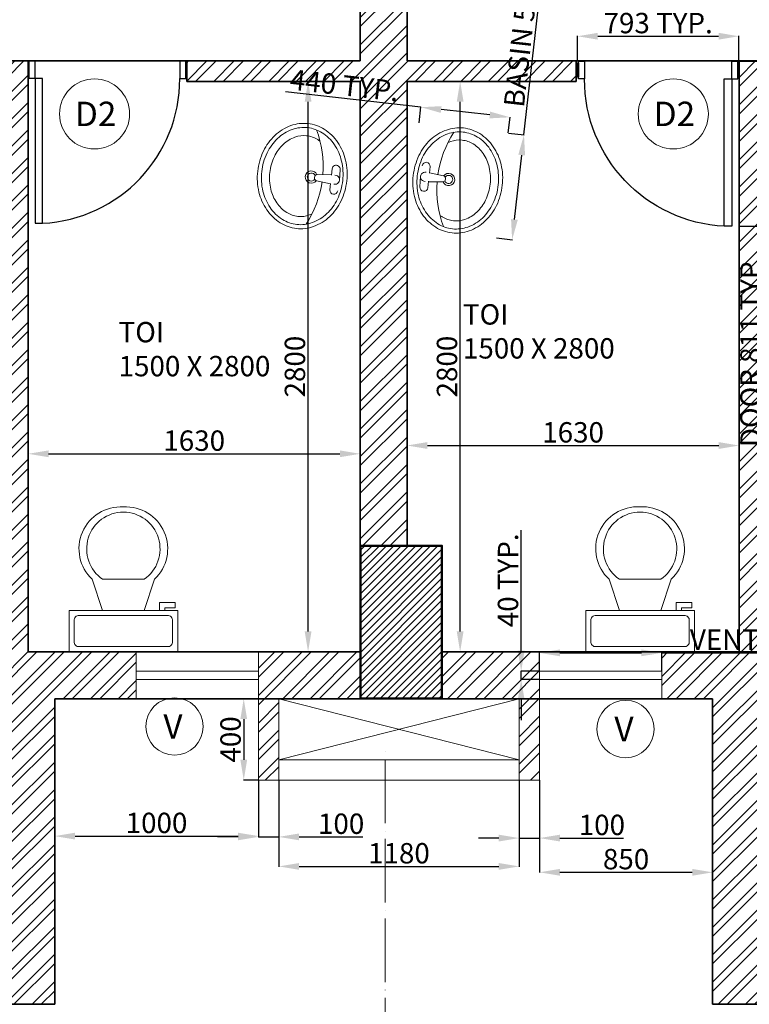
# Model space of a CAD drawing. Units: millimetres. Extents: x -3326 to 29338, y -16792 to 6002.
# Tile 15 of 21: x 21421 to 25002, y -12764 to -7931. Entities that reach past the tile are written whole.
import ezdxf

# ---------------------------------------------------------------- set-up
doc = ezdxf.new("R2010")
doc.units = ezdxf.units.MM
doc.header["$PDMODE"] = 35
doc.header["$PDSIZE"] = 5
doc.linetypes.add('ACAD_ISO04W100', pattern=[30, 24, -3, 0, -3])
for name, color, linetype, lineweight in [('A-ANNO-DIMS', 2, 'Continuous', 13), ('A-ANNO-SYMB', 7, 'Continuous', 18), ('A-AREA-IDEN', 7, 'Continuous', 18), ('A-COLS', 1, 'Continuous', 50), ('A-COLS-PATT', 251, 'Continuous', 13), ('A-DOOR', 3, 'Continuous', 25), ('A-FLOR-FIXT', 9, 'Continuous', 18), ('A-FLOR-SHFT', 8, 'Continuous', 18), ('A-GLAZ', 4, 'Continuous', 18), ('A-GRID', 8, 'ACAD_ISO04W100', 13), ('A-WALL', 7, 'Continuous', 35), ('A-WALL-PATT', 252, 'Continuous', 13)]:
    doc.layers.add(name, color=color, linetype=linetype, lineweight=lineweight)
doc.styles.get("Standard").update_dxf_attribs({"font": 'arial.ttf'})
doc.dimstyles.new('ISO-25', dxfattribs={"dimtxt": 100, "dimasz": 100, "dimexe": 1.25, "dimexo": 0.625, "dimtad": 1, "dimtxsty": 'Standard', "dimcen": 2.5, "dimadec": 0, "dimazin": 0, "dimtfac": 1, "dimtmove": 0, "dimatfit": 3, "dimfxl": 1, "dimarcsym": 0})

# ---------------------------------------------------------------- blocks, each defined once
blk = doc.blocks.new('A$C0CE462CD')
for p, q in [((860, 100), (860, 0)), ((860, 0), (893.9, 0))]:
    blk.add_line(p, q)
for points in [[(860, 100), (860, 920), (818.4, 920), (818.4, 100)], [(0, 10), (6.1, 10), (6.1, 90), (0, 90)], [(893.9, 10), (900, 10), (900, 90), (893.9, 90)]]:
    blk.add_lwpolyline(points, close=True)
for points in [[(6.1, 0), (40, 0), (40, 100), (6.1, 100)], [(6.1, 100), (6.1, 0)], [(860, 100), (893.9, 100), (893.9, 0)]]:
    blk.add_lwpolyline(points)
blk.add_arc((859.1, 101.9), 819.1, 92.8508, 180.1309)
blk = doc.blocks.new('*U5')
for p, q in [((9.5, -6), (9.5, -2)), ((-10, -8.5), (-8, -8.5)), ((-10, -9.5), (-10, -8.5)), ((-7, -9.5), (-10, -9.5)), ((-8, -8.5), (-8, -8)), ((-7, -8), (-7, -9.5)), ((-4, -8), (-6, -14)), ((4, -8), (6, -14)), ((4, -14), (-4, -14))]:
    blk.add_line(p, q)
blk.add_lwpolyline([(10.5, -8), (10.5, 0), (-10.5, 0), (-10.5, -8)], close=True)
for points in [[(8.5, -1), (-8.5, -1)], [(-9.5, -2), (-9.5, -6)], [(-8.5, -7), (8.5, -7)]]:
    blk.add_lwpolyline(points)
for centre, radius, start, end in [((-8.625, -1.875), 0.8839, 81.8699, 188.1301), ((8.625, -1.875), 0.8839, 351.8699, 98.1301), ((-8.625, -6.125), 0.8839, 171.869898, 278.1301), ((8.625, -6.125), 0.8839, 261.8699, 8.1301), ((-0.4772, -19.9188), 8.0953, 133.01722, 273.38), ((0.0374, -19.8731), 7.127, 124.50543, 269.7), ((-0.0373, -19.8731), 7.127, 270.3, 55.4946), ((0.4773, -19.9188), 8.0953, 266.62, 46.9828)]:
    blk.add_arc(centre, radius, start, end)
blk = doc.blocks.new('A$C6B943AC5')
for p, q in [((0.207, 0.401), (0.2589, 0.4042)), ((0.2071, 0.362), (0.2386, 0.3621)), ((0.2361, 0.3625), (0.2439, 0.2926)), ((0.2809, 0.3627), (0.2736, 0.2927)), ((0.3111, 0.3624), (0.2796, 0.3623))]:
    blk.add_line(p, q)
for points in [[(0.518, 0.2209, -0.113917), (0.4993, 0.1385, -0.1036), (0.4427, 0.0651, -0.091717), (0.3606, 0.0176, -0.084781), (0.2598, 0, -0.084781), (0.1587, 0.0169, -0.091717), (0.0764, 0.0638, -0.1036), (0.0193, 0.1368, -0.113917), (0, 0.2191, -0.113917), (0.0187, 0.3015, -0.1036), (0.0753, 0.3749, -0.091717), (0.1574, 0.4224, -0.084781), (0.2582, 0.44, -0.084781), (0.3592, 0.4231, -0.091717), (0.4416, 0.3762, -0.1036), (0.4987, 0.3032, -0.113917)], [(0.498, 0.2208, -0.113917), (0.4813, 0.1472, -0.1036), (0.4297, 0.0803, -0.091717), (0.3539, 0.0364, -0.084781), (0.2597, 0.02, -0.084781), (0.1653, 0.0358, -0.091717), (0.0893, 0.0791, -0.1036), (0.0372, 0.1457, -0.113917), (0.02, 0.2192, -0.113917), (0.0367, 0.2928, -0.1036), (0.0883, 0.3597, -0.091717), (0.1641, 0.4036, -0.084781), (0.2583, 0.42, -0.084781), (0.3527, 0.4042, -0.091717), (0.4287, 0.3609, -0.1036), (0.4808, 0.2943, -0.113917)]]:
    blk.add_lwpolyline(points, format="xyb", close=True)
for points in [[(0.458, 0.2207, -0.113917), (0.4453, 0.1646, -0.1036), (0.4037, 0.1107, -0.091717), (0.3405, 0.0741, -0.084781), (0.2595, 0.06, -0.084781), (0.1785, 0.0736, -0.091717), (0.1151, 0.1097, -0.1036), (0.0731, 0.1633, -0.113917), (0.06, 0.2193, -0.113917), (0.0727, 0.2754, -0.020517), (0.0792, 0.2874, -0.091717)], [(0.4384, 0.2886, -0.020517), (0.4449, 0.2767, -0.113917), (0.458, 0.2207, -0.113917)]]:
    blk.add_lwpolyline(points, format="xyb")
for centre, radius, start, end in [((0.207, 0.3815), 0.0195, 90.197, 270.197), ((0.259, 0.3817), 0.0225, 354.0815, 186.3125), ((0.311, 0.3819), 0.0195, 270.197, 90.197), ((0.2604, -0.2004), 0.5204, 92.1543, 116.7762), ((0.2588, 0.265), 0.03, 119.152, 61.242), ((0.2587, 0.295), 0.015, 189.3922, 351.0017), ((0.2604, -0.2004), 0.5204, 63.6178, 88.2397), ((0.2588, 0.265), 0.02, 116.5813, 63.8126)]:
    blk.add_arc(centre, radius, start, end)
blk = doc.blocks.new('*D17')
at = {"layer": 'A-ANNO-DIMS', "color": 0, "lineweight": -2, "transparency": 16777216}
for p, q in [((22592.3, -11664.6), (22592.3, -11943.5)), ((22692.3, -11664.6), (22692.3, -11943.5)), ((22492.3, -11942.2), (22392.3, -11942.2)), ((22592.3, -11942.2), (22692.3, -11942.2)), ((22792.3, -11942.2), (23104.7, -11942.2))]:
    blk.add_line(p, q, dxfattribs=at)
at = {"layer": 'A-ANNO-DIMS', "color": 0, "transparency": 16777216}
for points in [[(22492.3, -11925.6), (22492.3, -11958.9), (22592.3, -11942.2)], [(22792.3, -11925.6), (22792.3, -11958.9), (22692.3, -11942.2)]]:
    blk.add_solid(points, dxfattribs=at)
at = {"layer": 'Defpoints', "color": 0, "transparency": 16777216}
for p in [(22592.3, -11664), (22692.3, -11664), (22692.3, -11942.2)]:
    blk.add_point(p, dxfattribs=at)
at = {"layer": 'A-ANNO-DIMS', "color": 0, "transparency": 16777216, "insert": (22998.5, -11890.6), "char_height": 100, "attachment_point": 5}
blk.add_mtext('100', dxfattribs=at)
blk = doc.blocks.new('*D18')
at = {"layer": 'A-ANNO-DIMS', "color": 0, "lineweight": -2, "transparency": 16777216}
for p, q in [((23872.3, -11664.6), (23872.3, -11949.3)), ((23972.3, -11664.6), (23972.3, -11949.3)), ((23772.3, -11948), (23672.3, -11948)), ((23872.3, -11948), (23972.3, -11948)), ((24072.3, -11948), (24384.7, -11948))]:
    blk.add_line(p, q, dxfattribs=at)
at = {"layer": 'A-ANNO-DIMS', "color": 0, "transparency": 16777216}
for points in [[(23772.3, -11931.4), (23772.3, -11964.7), (23872.3, -11948)], [(24072.3, -11931.4), (24072.3, -11964.7), (23972.3, -11948)]]:
    blk.add_solid(points, dxfattribs=at)
at = {"layer": 'Defpoints', "color": 0, "transparency": 16777216}
for p in [(23872.3, -11664), (23972.3, -11664), (23972.3, -11948)]:
    blk.add_point(p, dxfattribs=at)
at = {"layer": 'A-ANNO-DIMS', "color": 0, "transparency": 16777216, "insert": (24278.5, -11896.4), "char_height": 100, "attachment_point": 5}
blk.add_mtext('100', dxfattribs=at)
blk = doc.blocks.new('*D19')
at = {"layer": 'A-ANNO-DIMS', "color": 0, "lineweight": -2, "transparency": 16777216}
for p, q in [((21592.3, -11798), (21592.3, -11939.6)), ((22592.3, -11798), (22592.3, -11939.6)), ((21692.3, -11938.3), (22492.3, -11938.3))]:
    blk.add_line(p, q, dxfattribs=at)
at = {"layer": 'A-ANNO-DIMS', "color": 0, "transparency": 16777216}
for points in [[(21692.3, -11921.7), (21692.3, -11955), (21592.3, -11938.3)], [(22492.3, -11921.7), (22492.3, -11955), (22592.3, -11938.3)]]:
    blk.add_solid(points, dxfattribs=at)
at = {"layer": 'Defpoints', "color": 0, "transparency": 16777216}
for p in [(21592.3, -11797.3), (22592.3, -11797.3), (22592.3, -11938.3)]:
    blk.add_point(p, dxfattribs=at)
at = {"layer": 'A-ANNO-DIMS', "color": 0, "transparency": 16777216, "insert": (22092.3, -11886.6), "char_height": 100, "attachment_point": 5}
blk.add_mtext('1000', dxfattribs=at)
blk = doc.blocks.new('*D20')
at = {"layer": 'A-ANNO-DIMS', "color": 0, "lineweight": -2, "transparency": 16777216}
for p, q in [((23972.3, -11807.6), (23972.3, -12117.4)), ((24822.3, -11807.6), (24822.3, -12117.4)), ((24072.3, -12116.1), (24722.3, -12116.1))]:
    blk.add_line(p, q, dxfattribs=at)
at = {"layer": 'A-ANNO-DIMS', "color": 0, "transparency": 16777216}
for points in [[(24072.3, -12099.5), (24072.3, -12132.8), (23972.3, -12116.1)], [(24722.3, -12099.5), (24722.3, -12132.8), (24822.3, -12116.1)]]:
    blk.add_solid(points, dxfattribs=at)
at = {"layer": 'Defpoints', "color": 0, "transparency": 16777216}
for p in [(23972.3, -11806.9), (24822.3, -11806.9), (24822.3, -12116.1)]:
    blk.add_point(p, dxfattribs=at)
at = {"layer": 'A-ANNO-DIMS', "color": 0, "transparency": 16777216, "insert": (24397.3, -12064.4), "char_height": 100, "attachment_point": 5}
blk.add_mtext('850', dxfattribs=at)
blk = doc.blocks.new('*D21')
at = {"layer": 'A-ANNO-DIMS', "color": 0, "lineweight": -2, "transparency": 16777216}
for p, q in [((22692.3, -11664.6), (22692.3, -12088.4)), ((23872.3, -11664.6), (23872.3, -12088.4)), ((22792.3, -12087.1), (23772.3, -12087.1))]:
    blk.add_line(p, q, dxfattribs=at)
at = {"layer": 'A-ANNO-DIMS', "color": 0, "transparency": 16777216}
for points in [[(22792.3, -12070.5), (22792.3, -12103.8), (22692.3, -12087.1)], [(23772.3, -12070.5), (23772.3, -12103.8), (23872.3, -12087.1)]]:
    blk.add_solid(points, dxfattribs=at)
at = {"layer": 'Defpoints', "color": 0, "transparency": 16777216}
for p in [(22692.3, -11664), (23872.3, -11664), (23872.3, -12087.1)]:
    blk.add_point(p, dxfattribs=at)
at = {"layer": 'A-ANNO-DIMS', "color": 0, "transparency": 16777216, "insert": (23282.3, -12035.5), "char_height": 100, "attachment_point": 5}
blk.add_mtext('1180', dxfattribs=at)
blk = doc.blocks.new('*D22')
at = {"layer": 'A-ANNO-DIMS', "color": 0, "lineweight": -2, "transparency": 16777216}
for p, q in [((21462.3, -10166), (21462.3, -10060.7)), ((21562.3, -10062), (22992.3, -10062)), ((23092.3, -10166), (23092.3, -10060.7))]:
    blk.add_line(p, q, dxfattribs=at)
at = {"layer": 'A-ANNO-DIMS', "color": 0, "transparency": 16777216}
for points in [[(21562.3, -10045.3), (21562.3, -10078.6), (21462.3, -10062)], [(22992.3, -10045.3), (22992.3, -10078.6), (23092.3, -10062)]]:
    blk.add_solid(points, dxfattribs=at)
at = {"layer": 'Defpoints', "color": 0, "transparency": 16777216}
for p in [(23092.3, -10062), (21462.3, -10166.6), (23092.3, -10166.6)]:
    blk.add_point(p, dxfattribs=at)
at = {"layer": 'A-ANNO-DIMS', "color": 0, "transparency": 16777216, "insert": (22277.3, -10010.3), "char_height": 100, "attachment_point": 5}
blk.add_mtext('1630', dxfattribs=at)
blk = doc.blocks.new('*D23')
at = {"layer": 'A-ANNO-DIMS', "color": 0, "lineweight": -2, "transparency": 16777216}
for p, q in [((22667.3, -8234), (22837.6, -8234)), ((22836.3, -10934), (22836.3, -8334)), ((22751.8, -11034), (22837.6, -11034))]:
    blk.add_line(p, q, dxfattribs=at)
at = {"layer": 'A-ANNO-DIMS', "color": 0, "transparency": 16777216}
for points in [[(22819.7, -8334), (22853, -8334), (22836.3, -8234)], [(22819.7, -10934), (22853, -10934), (22836.3, -11034)]]:
    blk.add_solid(points, dxfattribs=at)
at = {"layer": 'Defpoints', "color": 0, "transparency": 16777216}
for p in [(22666.7, -8234), (22836.3, -8234), (22751.1, -11034)]:
    blk.add_point(p, dxfattribs=at)
at = {"layer": 'A-ANNO-DIMS', "color": 0, "transparency": 16777216, "insert": (22784.6, -9634), "char_height": 100, "attachment_point": 5, "rotation": 90}
blk.add_mtext('2800', dxfattribs=at)
blk = doc.blocks.new('*D24')
at = {"layer": 'A-ANNO-DIMS', "color": 0, "lineweight": -2, "transparency": 16777216}
for p, q in [((23669.4, -8234), (23581.6, -8234)), ((23582.8, -10934), (23582.8, -8334)), ((23669.4, -11034), (23581.6, -11034))]:
    blk.add_line(p, q, dxfattribs=at)
at = {"layer": 'A-ANNO-DIMS', "color": 0, "transparency": 16777216}
for points in [[(23566.1, -8334), (23599.5, -8334), (23582.8, -8234)], [(23566.1, -10934), (23599.5, -10934), (23582.8, -11034)]]:
    blk.add_solid(points, dxfattribs=at)
at = {"layer": 'Defpoints', "color": 0, "transparency": 16777216}
for p in [(23582.8, -8234), (23670.1, -8234), (23670.1, -11034)]:
    blk.add_point(p, dxfattribs=at)
at = {"layer": 'A-ANNO-DIMS', "color": 0, "transparency": 16777216, "insert": (23531.1, -9634), "char_height": 100, "attachment_point": 5, "rotation": 90}
blk.add_mtext('2800', dxfattribs=at)
blk = doc.blocks.new('*D25')
at = {"layer": 'A-ANNO-DIMS', "color": 0, "lineweight": -2, "transparency": 16777216}
for p, q in [((23322.3, -10020.7), (23322.3, -10020.1)), ((23422.3, -10021.3), (24852.3, -10021.3)), ((24952.3, -10020.7), (24952.3, -10020.1))]:
    blk.add_line(p, q, dxfattribs=at)
at = {"layer": 'A-ANNO-DIMS', "color": 0, "transparency": 16777216}
for points in [[(23422.3, -10004.6), (23422.3, -10038), (23322.3, -10021.3)], [(24852.3, -10004.6), (24852.3, -10038), (24952.3, -10021.3)]]:
    blk.add_solid(points, dxfattribs=at)
at = {"layer": 'Defpoints', "color": 0, "transparency": 16777216}
for p in [(23322.3, -10021.3), (24952.3, -10021.3), (24952.3, -10021.3)]:
    blk.add_point(p, dxfattribs=at)
at = {"layer": 'A-ANNO-DIMS', "color": 0, "transparency": 16777216, "insert": (24137.3, -9969.6), "char_height": 100, "attachment_point": 5}
blk.add_mtext('1630', dxfattribs=at)
blk = doc.blocks.new('*D67')
at = {"layer": 'A-ANNO-DIMS', "color": 0, "lineweight": -2, "transparency": 16777216}
for p, q in [((22591.7, -11264), (22519.2, -11264)), ((22520.4, -11364), (22520.4, -11564)), ((22591.7, -11664), (22519.2, -11664))]:
    blk.add_line(p, q, dxfattribs=at)
at = {"layer": 'A-ANNO-DIMS', "color": 0, "transparency": 16777216}
for points in [[(22503.8, -11364), (22537.1, -11364), (22520.4, -11264)], [(22503.8, -11564), (22537.1, -11564), (22520.4, -11664)]]:
    blk.add_solid(points, dxfattribs=at)
at = {"layer": 'Defpoints', "color": 0, "transparency": 16777216}
for p in [(22592.3, -11264), (22520.4, -11664), (22592.3, -11664)]:
    blk.add_point(p, dxfattribs=at)
at = {"layer": 'A-ANNO-DIMS', "color": 0, "transparency": 16777216, "insert": (22468.7, -11464), "char_height": 100, "attachment_point": 5, "rotation": 90}
blk.add_mtext('400', dxfattribs=at)
blk = doc.blocks.new('TAG-D2')
blk.add_circle((172, 172), 172)
at = {"insert": (75.7, 232.2), "char_height": 120, "attachment_point": 1}
blk.add_mtext_dynamic_manual_height_columns('D2', width=130.724, gutter_width=12.5, heights=[0], dxfattribs=at)
blk = doc.blocks.new('TAG-V')
blk.add_circle((140.7, 140.7), 140.7)
at = {"insert": (85.8, 200.7), "char_height": 120, "attachment_point": 1}
blk.add_mtext_dynamic_manual_height_columns('V', width=129.836, gutter_width=12.5, heights=[0], dxfattribs=at)
blk = doc.blocks.new('GLAZ-600x40')
for p, q in [((600, 40), (0, 40)), ((600, 0), (0, 0))]:
    blk.add_line(p, q)
blk = doc.blocks.new('*D189')
at = {"layer": 'A-ANNO-DIMS', "color": 0, "lineweight": -2, "transparency": 16777216}
for p, q in [((24952.2, -8134.2), (25074.5, -8134.2)), ((25073.2, -8234.2), (25073.2, -8845.3)), ((24952.2, -8945.3), (25074.5, -8945.3)), ((25073.2, -8945.3), (25073.2, -10063.9))]:
    blk.add_line(p, q, dxfattribs=at)
at = {"layer": 'A-ANNO-DIMS', "color": 0, "transparency": 16777216}
for points in [[(25056.6, -8234.2), (25089.9, -8234.2), (25073.2, -8134.2)], [(25056.6, -8845.3), (25089.9, -8845.3), (25073.2, -8945.3)]]:
    blk.add_solid(points, dxfattribs=at)
at = {"layer": 'Defpoints', "color": 0, "transparency": 16777216}
for p in [(24951.6, -8134.2), (24951.6, -8945.3), (25073.2, -8945.3)]:
    blk.add_point(p, dxfattribs=at)
at = {"layer": 'A-ANNO-DIMS', "color": 0, "transparency": 16777216, "insert": (25020.9, -9554.6), "char_height": 100, "attachment_point": 5, "rotation": 90}
blk.add_mtext('DOOR 811 TYP.', dxfattribs=at)
blk = doc.blocks.new('*D190')
at = {"layer": 'A-ANNO-DIMS', "color": 0, "lineweight": -2, "transparency": 16777216}
for p, q in [((24158.2, -8133.6), (24158.2, -8011.3)), ((24258.2, -8012.6), (24851.6, -8012.6)), ((24951.6, -8133.6), (24951.6, -8011.3))]:
    blk.add_line(p, q, dxfattribs=at)
at = {"layer": 'A-ANNO-DIMS', "color": 0, "transparency": 16777216}
for points in [[(24258.2, -7995.9), (24258.2, -8029.2), (24158.2, -8012.6)], [(24851.6, -7995.9), (24851.6, -8029.2), (24951.6, -8012.6)]]:
    blk.add_solid(points, dxfattribs=at)
at = {"layer": 'Defpoints', "color": 0, "transparency": 16777216}
for p in [(24951.6, -8012.6), (24158.2, -8134.2), (24951.6, -8134.2)]:
    blk.add_point(p, dxfattribs=at)
at = {"layer": 'A-ANNO-DIMS', "color": 0, "transparency": 16777216, "insert": (24554.9, -7960.9), "char_height": 100, "attachment_point": 5}
blk.add_mtext('793 TYP.', dxfattribs=at)
blk = doc.blocks.new('*D205')
at = {"layer": 'A-ANNO-DIMS', "color": 0, "lineweight": -2, "transparency": 16777216}
for p, q in [((23972.3, -11128.3), (23972.3, -11037.7)), ((24072.3, -11039), (24472.3, -11039)), ((24572.3, -11128.3), (24572.3, -11037.7)), ((24572.3, -11039), (25654.6, -11039))]:
    blk.add_line(p, q, dxfattribs=at)
at = {"layer": 'A-ANNO-DIMS', "color": 0, "transparency": 16777216}
for points in [[(24072.3, -11022.3), (24072.3, -11055.6), (23972.3, -11039)], [(24472.3, -11022.3), (24472.3, -11055.6), (24572.3, -11039)]]:
    blk.add_solid(points, dxfattribs=at)
at = {"layer": 'Defpoints', "color": 0, "transparency": 16777216}
for p in [(24572.3, -11039), (23972.3, -11129), (24572.3, -11129)]:
    blk.add_point(p, dxfattribs=at)
at = {"layer": 'A-ANNO-DIMS', "color": 0, "transparency": 16777216, "insert": (25163.4, -10987.3), "char_height": 100, "attachment_point": 5}
blk.add_mtext('VENT 600 TYP.', dxfattribs=at)
blk = doc.blocks.new('*D206')
at = {"layer": 'A-ANNO-DIMS', "color": 0, "lineweight": -2, "transparency": 16777216}
for p, q in [((23882.3, -11029), (23882.3, -10436.9)), ((23971.7, -11129), (23881.1, -11129)), ((23882.3, -11169), (23882.3, -11129)), ((23971.7, -11169), (23881.1, -11169)), ((23882.3, -11269), (23882.3, -11369))]:
    blk.add_line(p, q, dxfattribs=at)
at = {"layer": 'A-ANNO-DIMS', "color": 0, "transparency": 16777216}
for points in [[(23865.6, -11029), (23899, -11029), (23882.3, -11129)], [(23865.6, -11269), (23899, -11269), (23882.3, -11169)]]:
    blk.add_solid(points, dxfattribs=at)
at = {"layer": 'Defpoints', "color": 0, "transparency": 16777216}
for p in [(23882.3, -11129), (23972.3, -11129), (23972.3, -11169)]:
    blk.add_point(p, dxfattribs=at)
at = {"layer": 'A-ANNO-DIMS', "color": 0, "transparency": 16777216, "insert": (23830.6, -10682.9), "char_height": 100, "attachment_point": 5, "rotation": 90}
blk.add_mtext('40 TYP.', dxfattribs=at)
blk = doc.blocks.new('*D215')
at = {"layer": 'A-ANNO-DIMS', "color": 0, "lineweight": -2, "transparency": 16777216}
for p, q in [((23896.1, -8496.3), (24021.7, -7384)), ((23819.5, -8487.6), (23897.4, -8496.4)), ((23849.2, -8911.8), (23884.9, -8595.6)), ((23761.4, -9002.6), (23839.2, -9011.3))]:
    blk.add_line(p, q, dxfattribs=at)
at = {"layer": 'A-ANNO-DIMS', "color": 0, "transparency": 16777216}
for points in [[(23868.3, -8593.8), (23901.5, -8597.5), (23896.1, -8496.3)], [(23832.6, -8910), (23865.8, -8913.7), (23838, -9011.2)]]:
    blk.add_solid(points, dxfattribs=at)
at = {"layer": 'Defpoints', "color": 0, "transparency": 16777216}
for p in [(23818.9, -8487.6), (23896.1, -8496.3), (23760.8, -9002.5)]:
    blk.add_point(p, dxfattribs=at)
at = {"layer": 'A-ANNO-DIMS', "color": 0, "transparency": 16777216, "insert": (23912.5, -7884.6), "char_height": 100, "attachment_point": 5, "rotation": 83.5597}
blk.add_mtext('BASIN 518 TYP.', dxfattribs=at)
blk = doc.blocks.new('*D216')
at = {"layer": 'A-ANNO-DIMS', "color": 0, "lineweight": -2, "transparency": 16777216}
for p, q in [((23390.1, -8360.9), (22724.6, -8285.8)), ((23381.5, -8437.6), (23390.3, -8359.7)), ((23728.2, -8399.1), (23489.5, -8372.2)), ((23818.9, -8486.9), (23827.7, -8409.1))]:
    blk.add_line(p, q, dxfattribs=at)
at = {"layer": 'A-ANNO-DIMS', "color": 0, "transparency": 16777216}
for points in [[(23491.4, -8355.6), (23487.6, -8388.7), (23390.1, -8360.9)], [(23730.1, -8382.5), (23726.4, -8415.7), (23827.6, -8410.3)]]:
    blk.add_solid(points, dxfattribs=at)
at = {"layer": 'Defpoints', "color": 0, "transparency": 16777216}
for p in [(23390.1, -8360.9), (23381.4, -8438.2), (23818.9, -8487.6)]:
    blk.add_point(p, dxfattribs=at)
at = {"layer": 'A-ANNO-DIMS', "color": 0, "transparency": 16777216, "insert": (23013.5, -8266.4), "char_height": 100, "attachment_point": 5, "rotation": 353.5597}
blk.add_mtext('440 TYP.', dxfattribs=at)

msp = doc.modelspace()

# ---------------------------------------------------------------- hatches: boundary and pattern name
at = {"layer": 'A-COLS-PATT'}
h = msp.add_hatch(dxfattribs=at)
h.set_pattern_fill('ANSI31', color=256, scale=8)
h.set_pattern_definition([(45, (-18945.38, -343.67), (-17.960512, 17.960512), [])])
h.paths.add_polyline_path([(23493.251, -10513.206), (23093.251, -10513.206), (23093.251, -11263.206), (23493.251, -11263.206)])
at = {"layer": 'A-WALL-PATT'}
h = msp.add_hatch(dxfattribs=at)
h.set_pattern_fill('ANSI32', color=256, scale=10)
h.set_pattern_definition([(45, (-10476.65, 1e-12), (-67.35192, 67.35192), []), (45, (-10431.74, 1e-12), (-67.35192, 67.35192), [])])
h.paths.add_polyline_path([(29282.301, -7283.952), (28882.301, -7283.952), (28882.301, -7383.952), (29052.301, -7383.952), (29052.301, -10763.952), (29282.301, -10763.952)])
h.paths.add_polyline_path([(29282.301, -11263.952), (29052.301, -11263.952), (29052.301, -12763.952), (29282.301, -12763.952)])
h.paths.add_polyline_path([(25052.301, -11263.952), (25652.301, -11263.952), (25652.301, -11123.904), (25652.289, -11123.904), (25652.289, -11033.952), (25052.301, -11033.952), (24572.301, -11033.952), (24572.301, -11263.952), (24822.301, -11263.952), (24822.301, -12763.952), (25052.301, -12763.952)])
h.paths.add_polyline_path([(26902.301, -11033.952), (26552.301, -11033.952), (26552.301, -11263.952), (26902.301, -11263.952)])
h.paths.add_polyline_path([(21992.301, -6683.952), (21362.301, -6683.952), (17512.301, -6683.952), (17512.301, -6783.952), (21362.301, -6783.952), (21992.301, -6783.952)])
h.paths.add_polyline_path([(17512.301, -7283.952), (17282.301, -7283.952), (17282.301, -12163.952), (17512.301, -12163.952), (17512.301, -11263.952), (18112.301, -11263.952), (18112.301, -11033.952), (17512.301, -11033.952)])
h.paths.add_polyline_path([(21462.301, -8211.864), (21462.064, -8211.864), (21462.064, -8142.609), (21462.301, -8133.952), (21362.301, -8133.952), (21362.301, -8233.952), (21362.301, -11033.952), (21162.301, -11033.952), (21162.301, -11263.952), (21362.301, -11263.952), (21362.301, -12763.952), (21592.301, -12763.952), (21592.301, -11263.952), (21992.301, -11263.952), (21992.301, -11033.952), (21592.301, -11033.952), (21462.301, -11033.952)])
h.paths.add_polyline_path([(24152.301, -8133.952), (23322.301, -8133.952), (23322.301, -7433.952), (23092.301, -7433.952), (23092.301, -8133.952), (22241.021, -8133.952), (22241.021, -8142.609), (22241.182, -8142.609), (22241.182, -8211.864), (22241.021, -8233.952), (23092.301, -8233.952), (23092.301, -10513.206), (23322.301, -10513.206), (23322.301, -8233.952), (24152.301, -8233.952)])
h.paths.add_polyline_path([(25052.301, -8233.952), (25052.301, -8133.952), (24952.301, -8133.952), (24952.301, -11033.952), (25052.301, -11033.952)])
h.paths.add_polyline_path([(23972.301, -11033.952), (23493.251, -11033.952), (23493.251, -11263.952), (23972.301, -11263.952)])
h.paths.add_polyline_path([(23092.301, -11033.952), (22592.301, -11033.952), (22592.301, -11263.952), (23092.301, -11263.952)])
h.paths.add_polyline_path([(28882.301, -11033.952), (28702.301, -11033.952), (28702.301, -11263.952), (28882.301, -11263.952)])
h.paths.add_polyline_path([(17512.301, -3883.952), (17387.589, -3883.952), (17387.589, -3888.07), (17282.301, -3888.07), (17282.301, -6683.952), (17512.301, -6683.952)])
h.paths.add_polyline_path([(21462.301, -2183.952), (21362.301, -2183.952), (21362.301, -2383.952), (17282.301, -2383.952), (17282.301, -2483.952), (17512.301, -2483.952), (21462.301, -2483.952)])
h.paths.add_polyline_path([(17512.301, -2483.952), (17282.301, -2483.952), (17282.301, -2833.952), (17512.301, -2833.952)])
h.paths.add_polyline_path([(21462.301, 1866.048), (21992.301, 1866.048), (21992.301, 2096.048), (21592.301, 2096.048), (21592.301, 3596.048), (21362.301, 3596.048), (21362.301, 1866.048), (21362.301, -1283.952), (21462.301, -1283.952)])
h.paths.add_polyline_path([(17512.301, 1496.048), (17282.301, 1496.048), (17282.301, -1983.952), (17612.301, -1983.952), (17612.301, -1883.952), (17512.301, -1883.952)])
h.paths.add_polyline_path([(17512.301, 3596.048), (17282.301, 3596.048), (17282.301, 2096.048), (17512.301, 2096.048)])
h.paths.add_polyline_path([(18135.023, 2096.048), (17685.023, 2096.048), (17685.023, 1866.048), (18135.023, 1866.048), (18135.023, 1876.048), (18128.942, 1876.048), (18128.942, 1956.048), (18135.023, 1956.048)])
h.paths.add_polyline_path([(19385.023, 2096.048), (19035.023, 2096.048), (19035.023, 1866.048), (19385.023, 1866.048)])
h.paths.add_polyline_path([(21362.301, 2096.048), (21185.023, 2096.048), (21185.023, 1866.048), (21362.301, 1866.048)])
h.paths.add_polyline_path([(23092.301, 2096.048), (22592.301, 2096.048), (22592.301, 1866.048), (23092.301, 1866.048)])
h.paths.add_polyline_path([(23972.301, 2096.048), (23492.301, 2096.048), (23492.301, 1866.048), (23972.301, 1866.048)])
h.paths.add_polyline_path([(23972.301, 2496.048), (23872.301, 2496.048), (23872.301, 2096.048), (23972.301, 2096.048)])
h.paths.add_polyline_path([(22692.301, 2496.048), (22592.301, 2496.048), (22592.301, 2096.048), (22692.301, 2096.048)])
h.paths.add_polyline_path([(23322.301, 1346.048), (23092.301, 1346.048), (23092.301, -1733.952), (23322.301, -1733.952)])
h.paths.add_polyline_path([(23092.301, -933.952), (22262.301, -933.952), (22262.301, -1033.952), (23092.301, -1033.952)])
h.paths.add_polyline_path([(24952.301, -1433.952), (24952.301, -1733.952), (23492.301, -1733.952), (23492.301, -1833.952), (24952.301, -1833.952), (24952.301, -2483.952), (25052.301, -2483.952), (25052.301, -2466.23), (25049.26, -2466.23), (25049.26, -2386.23), (25049.941, -1433.952)])
h.paths.add_polyline_path([(22692.301, -11263.952), (22592.301, -11263.952), (22592.301, -11663.952), (22692.301, -11663.952)])
h.paths.add_polyline_path([(23972.301, -11263.952), (23872.301, -11263.952), (23872.301, -11663.952), (23972.301, -11663.952)])

# ---------------------------------------------------------------- linework, layer by layer
at = {"layer": 'A-COLS'}
msp.add_lwpolyline([(23093.251, -10513.206), (23493.251, -10513.206), (23493.251, -11263.206), (23093.251, -11263.206)], close=True, dxfattribs=at)
at = {"layer": 'A-FLOR-SHFT'}
for p, q in [((22592.301, -11263.952), (22592.301, -11663.952)), ((22692.301, -11663.952), (22692.301, -11263.952)), ((22692.301, -11563.952), (23872.301, -11263.952)), ((22692.301, -11263.952), (23872.301, -11563.952)), ((23872.301, -11663.952), (23872.301, -11263.952)), ((23972.301, -11263.952), (23972.301, -11663.952)), ((22692.301, -11563.952), (23872.301, -11563.952)), ((22592.301, -11663.952), (22692.301, -11663.952)), ((22692.301, -11663.952), (23872.301, -11663.952)), ((23972.301, -11663.952), (23872.301, -11663.952))]:
    msp.add_line(p, q, dxfattribs=at)
at = {"layer": 'A-GLAZ'}
for p, q in [((21992.301, -11263.952), (21992.301, -11033.952)), ((22592.301, -11263.952), (22592.301, -11033.952)), ((23972.301, -11263.952), (23972.301, -11033.952)), ((24572.301, -11263.952), (24572.301, -11033.952))]:
    msp.add_line(p, q, dxfattribs=at)
at = {"layer": 'A-GRID', "ltscale": 13}
msp.add_line((23214.966, -13434.889), (23214.966, -11505.956), dxfattribs=at)
at = {"layer": 'A-WALL'}
for p, q in [((23092.301, -6683.952), (23092.301, -8133.952)), ((23322.301, -7433.952), (23322.301, -8133.952)), ((23092.301, -8133.952), (21362.301, -8133.952)), ((21462.301, -8133.952), (21462.301, -11033.952)), ((22241.021, -8133.952), (22241.021, -8233.952)), ((25052.301, -8133.952), (23322.301, -8133.952)), ((24152.301, -8133.952), (24152.301, -8233.952)), ((24952.301, -8133.952), (24952.301, -11033.952)), ((23092.301, -8233.952), (22241.021, -8233.952)), ((23092.301, -8233.952), (23092.301, -11263.952)), ((24152.301, -8233.952), (23322.301, -8233.952)), ((23322.301, -8233.952), (23322.301, -10513.206)), ((21592.301, -11033.952), (21462.301, -11033.952)), ((23093.251, -11033.952), (21592.301, -11033.952)), ((25052.301, -11033.952), (23493.251, -11033.952)), ((24822.301, -11263.952), (21592.301, -11263.952)), ((21592.301, -11263.952), (21592.301, -12763.952)), ((24822.301, -11263.952), (24822.301, -12763.952)), ((21592.301, -12763.952), (21362.301, -12763.952)), ((25052.301, -12763.952), (24822.301, -12763.952))]:
    msp.add_line(p, q, dxfattribs=at)

# ---------------------------------------------------------------- block references
at = {"layer": 'A-ANNO-SYMB'}
for name, p in [('TAG-D2', (21615.986, -8565.925)), ('TAG-D2', (24457.219, -8565.925)), ('TAG-V', (22040.077, -11540.823)), ('TAG-V', (24254.098, -11553.549))]:
    msp.add_blockref(name, p, dxfattribs=at)
at = {"layer": 'A-DOOR', "rotation": 180}
for p, xscale, yscale, zscale in [((22241.182, -8133.952), 0.86568603647667, 0.86568603647667, 0.86568603647667), ((24158.171, -8134.238), -0.8815660776293341, 0.8815660776293341, 0.8815660776293341)]:
    msp.add_blockref('A$C0CE462CD', p, dxfattribs=dict(at, xscale=xscale, yscale=yscale, zscale=zscale))
at = {"layer": 'A-FLOR-FIXT'}
for name, p, xscale, yscale, zscale, rotation in [('A$C6B943AC5', (22617.964, -8416.762), 999.9999999999998, 999.9999999999998, 999.9999999999998, 263.5597085968623), ('A$C6B943AC5', (23760.645, -9002.373), 999.9999999999998, 999.9999999999998, 999.9999999999998, 83.55970859686228), ('*U5', (21929.394, -11033.718), 25.4, 25.4, 25.4, 180), ('*U5', (24465.957, -11033.654), 25.4, 25.4, 25.4, 180)]:
    msp.add_blockref(name, p, dxfattribs=dict(at, xscale=xscale, yscale=yscale, zscale=zscale, rotation=rotation))
at = {"layer": 'A-GLAZ'}
for p in [(21992.301, -11168.952), (23972.301, -11168.952)]:
    msp.add_blockref('GLAZ-600x40', p, dxfattribs=at)

# ---------------------------------------------------------------- texts
at = {"layer": 'A-AREA-IDEN', "char_height": 100, "attachment_point": 1}
for insert in [(23596.508, -9327.771), (21906.163, -9414.945)]:
    msp.add_mtext_dynamic_manual_height_columns('TOI\\P1500 X 2800', width=1168.90663, gutter_width=12.5, heights=[0], dxfattribs=dict(at, insert=insert))

# ---------------------------------------------------------------- dimensions: what is measured, and where the dimension line sits
at = {"layer": 'A-ANNO-DIMS'}
for base, p1, p2, angle, text, picture, middle in [((23896.114, -8496.279), (23760.751, -9002.484), (23818.876, -8487.561), 83.559709, 'BASIN <> TYP.', '*D215', (23912.499, -7884.594)), ((23390.139, -8360.942), (23818.876, -8487.561), (23381.42, -8438.181), 173.559709, '<> TYP.', '*D216', (23013.497, -8266.416)), ((25073.237, -8945.279), (24951.581, -8134.238), (24951.581, -8945.279), 270, 'DOOR <> TYP.', '*D189', (25020.872, -9554.601)), ((23882.301, -11128.952), (23972.301, -11168.952), (23972.301, -11128.952), 90, '<> TYP.', '*D206', (23830.618, -10682.931))]:
    dim = msp.add_linear_dim(base=base, p1=p1, p2=p2, angle=angle, text=text, dimstyle='ISO-25', override={"dimdec": 0, "dimlfac": 1, "dimrnd": 0, "dimzin": 0, "dimdsep": 46, "dimlunit": 2}, dxfattribs=at)
    dim.commit()
    dim.dimension.update_dxf_attribs({"geometry": picture, "text_midpoint": middle})
for base, p1, p2, text, picture, middle in [((24951.581, -8012.582), (24158.171, -8134.238), (24951.581, -8134.238), '<> TYP.', '*D190', (24554.876, -7960.865)), ((24572.301, -11038.952), (23972.301, -11128.952), (24572.301, -11128.952), 'VENT <> TYP.', '*D205', (25163.444, -10987.27))]:
    dim = msp.add_linear_dim(base=base, p1=p1, p2=p2, text=text, dimstyle='ISO-25', override={"dimdec": 0, "dimlfac": 1, "dimrnd": 0, "dimzin": 0, "dimdsep": 46, "dimlunit": 2}, dxfattribs=at)
    dim.commit()
    dim.dimension.update_dxf_attribs({"geometry": picture, "text_midpoint": middle})
for base, p1, p2, picture, middle in [((22836.331, -8233.952), (22751.148, -11033.952), (22666.661, -8233.952), '*D23', (22784.649, -9633.952)), ((23582.816, -8233.952), (23670.054, -11033.952), (23670.054, -8233.952), '*D24', (23531.134, -9633.952)), ((22520.423, -11663.952), (22592.301, -11263.952), (22592.301, -11663.952), '*D67', (22468.74, -11463.952))]:
    dim = msp.add_linear_dim(base=base, p1=p1, p2=p2, angle=90, dimstyle='ISO-25', override={"dimclrd": 0, "dimclre": 0, "dimclrt": 0}, dxfattribs=at)
    dim.commit()
    dim.dimension.update_dxf_attribs({"geometry": picture, "text_midpoint": middle})
for base, p1, p2, picture, middle in [((24952.301, -10021.301), (23322.301, -10021.301), (24952.301, -10021.301), '*D25', (24137.301, -9969.585)), ((23092.301, -10061.98), (21462.301, -10166.582), (23092.301, -10166.582), '*D22', (22277.301, -10010.263)), ((22692.301, -11942.248), (22592.301, -11663.952), (22692.301, -11663.952), '*D17', (22998.519, -11890.566)), ((23872.301, -12087.147), (22692.301, -11663.952), (23872.301, -11663.952), '*D21', (23282.301, -12035.464)), ((23972.301, -11948.044), (23872.301, -11663.952), (23972.301, -11663.952), '*D18', (24278.519, -11896.361)), ((22592.301, -11938.332), (21592.301, -11797.349), (22592.301, -11797.349), '*D19', (22092.301, -11886.649)), ((24822.301, -12116.127), (23972.301, -11806.935), (24822.301, -11806.935), '*D20', (24397.301, -12064.444))]:
    dim = msp.add_linear_dim(base=base, p1=p1, p2=p2, dimstyle='ISO-25', override={"dimclrd": 0, "dimclre": 0, "dimclrt": 0}, dxfattribs=at)
    dim.commit()
    dim.dimension.update_dxf_attribs({"geometry": picture, "text_midpoint": middle})

doc.saveas('drawing.dxf')
